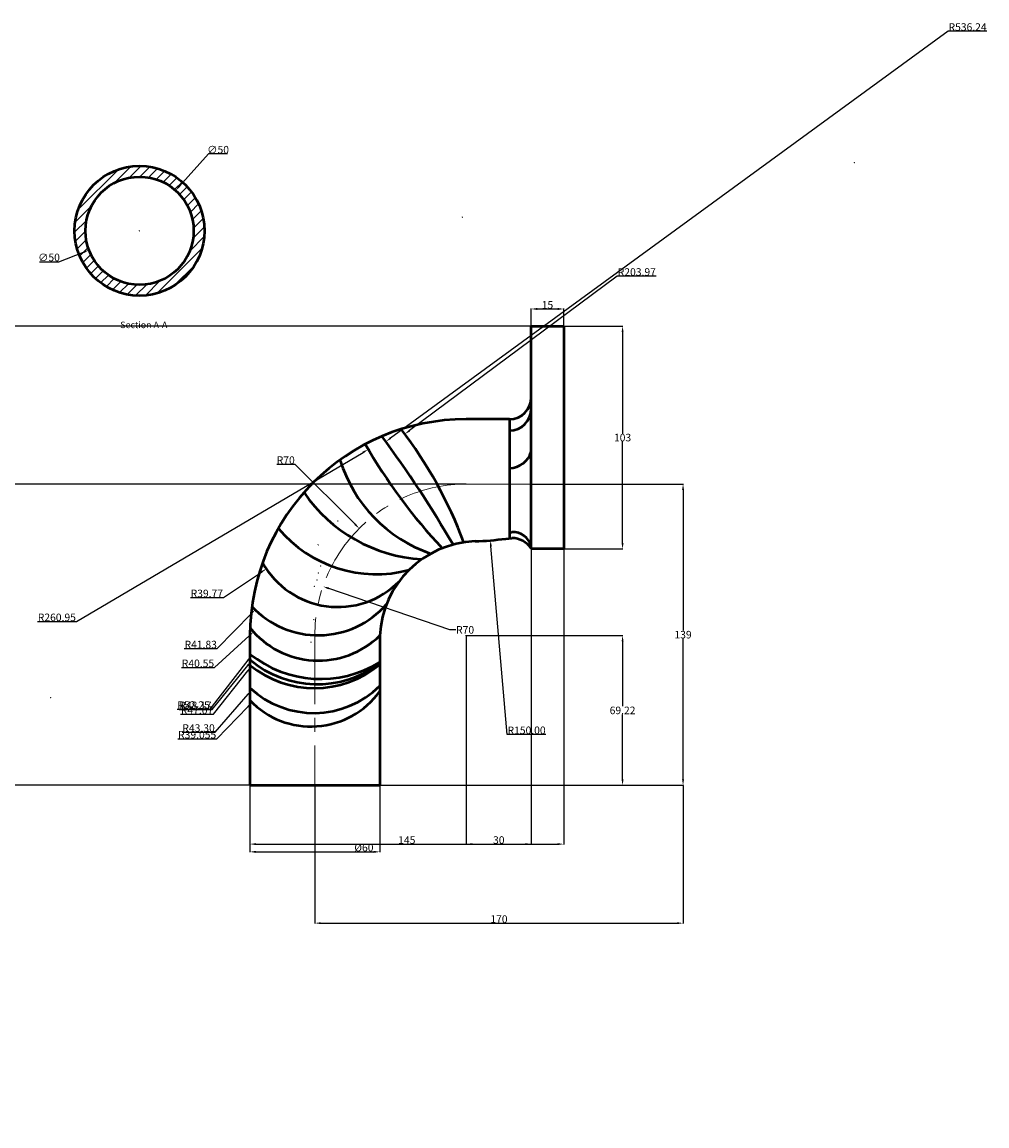
# Model space of a CAD drawing. Units: millimetres. Extents: x 795 to 1506, y 326 to 837.
# Tile 2 of 2: x 1060 to 1506, y 326 to 837. Entities that reach past the tile are written whole.
import ezdxf

# ---------------------------------------------------------------- set-up
doc = ezdxf.new("R2010")
doc.units = ezdxf.units.MM
doc.header["$MEASUREMENT"] = 0
doc.linetypes.add('CENTER', pattern=[50.8, 31.75, -6.35, 6.35, -6.35])
for name, color, linetype, lineweight in [('M-CNTR', 251, 'CENTER', 18), ('M-DIMS', 2, 'Continuous', 25), ('M-HATC', 8, 'Continuous', 18), ('M-OUTL', 7, 'Continuous', 50), ('M-TEXT', 7, 'Continuous', 25)]:
    doc.layers.add(name, color=color, linetype=linetype, lineweight=lineweight)
doc.styles.get("Standard").update_dxf_attribs({"font": 'arial.ttf'})
doc.dimstyles.get("Standard").update_dxf_attribs({"dimtxt": 3.5, "dimasz": 2.75, "dimexe": 0.18, "dimexo": 0.0625, "dimgap": 0.09, "dimtad": 1, "dimtih": 1, "dimtoh": 1, "dimdec": 0, "dimzin": 0, "dimdsep": 46, "dimtxsty": 'Standard', "dimcen": 0.09, "dimadec": 0, "dimazin": 0, "dimtfac": 1, "dimtdec": 0, "dimtofl": 0, "dimtmove": 0, "dimatfit": 3, "dimfxl": 1, "dimtolj": 1, "dimtzin": 0, "dimarcsym": 0})

# ---------------------------------------------------------------- blocks, each defined once
blk = doc.blocks.new('*D4')
at = {"layer": 'Defpoints', "color": 0, "transparency": 16777216}
for p in [(1295.11, 622.98), (1225.11, 483.77), (1365.27, 483.77)]:
    blk.add_point(p, dxfattribs=at)
at = {"layer": 'M-DIMS', "color": 0, "lineweight": -2, "transparency": 16777216}
for p, q in [((1295.17, 622.98), (1365.45, 622.98)), ((1365.27, 620.23), (1365.27, 555.25)), ((1365.27, 486.52), (1365.27, 551.5)), ((1225.17, 483.77), (1365.45, 483.77))]:
    blk.add_line(p, q, dxfattribs=at)
at = {"layer": 'M-DIMS', "color": 0, "transparency": 16777216}
for points in [[(1364.81, 620.23), (1365.72, 620.23), (1365.27, 622.98)], [(1364.81, 486.52), (1365.72, 486.52), (1365.27, 483.77)]]:
    blk.add_solid(points, dxfattribs=at)
at = {"layer": 'M-DIMS', "color": 0, "transparency": 16777216, "insert": (1365.27, 553.37), "char_height": 3.5, "attachment_point": 5}
blk.add_mtext('\\A1;139', dxfattribs=at)
blk = doc.blocks.new('*D5')
at = {"layer": 'Defpoints', "color": 0, "transparency": 16777216}
for p in [(1165.11, 483.77), (1225.11, 483.77), (1225.11, 452.98)]:
    blk.add_point(p, dxfattribs=at)
at = {"layer": 'M-DIMS', "color": 0, "lineweight": -2, "transparency": 16777216}
for p, q in [((1165.11, 483.7), (1165.11, 452.8)), ((1225.11, 483.7), (1225.11, 452.8)), ((1167.86, 452.98), (1222.36, 452.98))]:
    blk.add_line(p, q, dxfattribs=at)
at = {"layer": 'M-DIMS', "color": 0, "transparency": 16777216}
for points in [[(1167.86, 453.43), (1167.86, 452.52), (1165.11, 452.98)], [(1222.36, 453.43), (1222.36, 452.52), (1225.11, 452.98)]]:
    blk.add_solid(points, dxfattribs=at)
at = {"layer": 'M-DIMS', "color": 0, "transparency": 16777216, "insert": (1217.78, 454.95), "char_height": 3.5, "attachment_point": 5}
blk.add_mtext('\\A1;%%C60', dxfattribs=at)
blk = doc.blocks.new('*D6')
at = {"layer": 'Defpoints', "color": 0, "transparency": 16777216}
for p in [(1195.11, 483.77), (1365.27, 483.77), (1365.27, 420.02)]:
    blk.add_point(p, dxfattribs=at)
at = {"layer": 'M-DIMS', "color": 0, "lineweight": -2, "transparency": 16777216}
for p, q in [((1195.11, 483.7), (1195.11, 419.84)), ((1365.27, 483.7), (1365.27, 419.84)), ((1197.86, 420.02), (1362.52, 420.02))]:
    blk.add_line(p, q, dxfattribs=at)
at = {"layer": 'M-DIMS', "color": 0, "transparency": 16777216}
for points in [[(1197.86, 420.47), (1197.86, 419.56), (1195.11, 420.02)], [(1362.52, 420.47), (1362.52, 419.56), (1365.27, 420.02)]]:
    blk.add_solid(points, dxfattribs=at)
at = {"layer": 'M-DIMS', "color": 0, "transparency": 16777216, "insert": (1280.19, 421.89), "char_height": 3.5, "attachment_point": 5}
blk.add_mtext('\\A1;170', dxfattribs=at)
blk = doc.blocks.new('*D7')
at = {"layer": 'Defpoints', "color": 0, "transparency": 16777216}
for p in [(1310.11, 703.93), (1295.11, 695.98), (1310.11, 695.98)]:
    blk.add_point(p, dxfattribs=at)
at = {"layer": 'M-DIMS', "color": 0, "lineweight": -2, "transparency": 16777216}
for p, q in [((1295.11, 696.04), (1295.11, 704.11)), ((1297.86, 703.93), (1307.36, 703.93)), ((1310.11, 696.04), (1310.11, 704.11))]:
    blk.add_line(p, q, dxfattribs=at)
at = {"layer": 'M-DIMS', "color": 0, "transparency": 16777216}
for points in [[(1297.86, 704.39), (1297.86, 703.47), (1295.11, 703.93)], [(1307.36, 704.39), (1307.36, 703.47), (1310.11, 703.93)]]:
    blk.add_solid(points, dxfattribs=at)
at = {"layer": 'M-DIMS', "color": 0, "transparency": 16777216, "insert": (1302.61, 705.81), "char_height": 3.5, "attachment_point": 5}
blk.add_mtext('\\A1;15', dxfattribs=at)
blk = doc.blocks.new('*D16')
at = {"layer": 'Defpoints', "color": 0, "transparency": 16777216}
for p in [(1130.77, 758.69), (1097.42, 721.44)]:
    blk.add_point(p, dxfattribs=at)
at = {"layer": 'M-DIMS', "color": 0, "lineweight": -2, "transparency": 16777216}
for p, q in [((1145.89, 775.58), (1132.6, 760.74)), ((1154.79, 775.58), (1145.89, 775.58)), ((1114.01, 740.07), (1114.19, 740.07)), ((1114.1, 739.98), (1114.1, 740.16))]:
    blk.add_line(p, q, dxfattribs=at)
at = {"layer": 'M-DIMS', "color": 0, "transparency": 16777216}
blk.add_solid([(1132.26, 761.05), (1132.95, 760.44), (1130.77, 758.69)], dxfattribs=at)
at = {"layer": 'M-DIMS', "color": 0, "transparency": 16777216, "insert": (1150.39, 777.56), "char_height": 3.5, "attachment_point": 5}
blk.add_mtext('\\A1;∅50', dxfattribs=at)
blk = doc.blocks.new('*D17')
at = {"layer": 'Defpoints', "color": 0, "transparency": 16777216}
for p in [(1198.88, 575.65), (1265.11, 552.98)]:
    blk.add_point(p, dxfattribs=at)
at = {"layer": 'M-DIMS', "color": 0, "lineweight": -2, "transparency": 16777216}
for p, q in [((1257.53, 555.58), (1201.49, 574.76)), ((1260.28, 555.58), (1257.53, 555.58))]:
    blk.add_line(p, q, dxfattribs=at)
at = {"layer": 'M-DIMS', "color": 0, "transparency": 16777216}
blk.add_solid([(1201.63, 575.2), (1201.34, 574.33), (1198.88, 575.65)], dxfattribs=at)
at = {"layer": 'M-DIMS', "color": 0, "transparency": 16777216, "insert": (1264.54, 555.58), "char_height": 3.5, "attachment_point": 5}
blk.add_mtext('\\A1;R70', dxfattribs=at)
blk = doc.blocks.new('*D24')
at = {"layer": 'Defpoints', "color": 0, "transparency": 16777216}
for p in [(1310.11, 695.98), (1310.11, 592.98), (1337.31, 592.98)]:
    blk.add_point(p, dxfattribs=at)
at = {"layer": 'M-DIMS', "color": 0, "lineweight": -2, "transparency": 16777216}
for p, q in [((1310.17, 695.98), (1337.49, 695.98)), ((1337.31, 693.23), (1337.31, 646.36)), ((1337.31, 595.73), (1337.31, 642.6)), ((1310.17, 592.98), (1337.49, 592.98))]:
    blk.add_line(p, q, dxfattribs=at)
at = {"layer": 'M-DIMS', "color": 0, "transparency": 16777216}
for points in [[(1336.85, 693.23), (1337.77, 693.23), (1337.31, 695.98)], [(1336.85, 595.73), (1337.77, 595.73), (1337.31, 592.98)]]:
    blk.add_solid(points, dxfattribs=at)
at = {"layer": 'M-DIMS', "color": 0, "transparency": 16777216, "insert": (1337.31, 644.48), "char_height": 3.5, "attachment_point": 5}
blk.add_mtext('\\A1;103', dxfattribs=at)
blk = doc.blocks.new('*D25')
at = {"layer": 'Defpoints', "color": 0, "transparency": 16777216}
for p in [(1310.11, 695.98), (824.22, 622.98), (1265.11, 622.98)]:
    blk.add_point(p, dxfattribs=at)
at = {"layer": 'M-DIMS', "color": 0, "lineweight": -2, "transparency": 16777216}
for p, q in [((1310.05, 695.98), (824.04, 695.98)), ((824.22, 693.23), (824.22, 661.36)), ((824.22, 625.73), (824.22, 657.6)), ((1265.05, 622.98), (824.04, 622.98))]:
    blk.add_line(p, q, dxfattribs=at)
at = {"layer": 'M-DIMS', "color": 0, "transparency": 16777216}
for points in [[(823.76, 693.23), (824.68, 693.23), (824.22, 695.98)], [(823.76, 625.73), (824.68, 625.73), (824.22, 622.98)]]:
    blk.add_solid(points, dxfattribs=at)
at = {"layer": 'M-DIMS', "color": 0, "transparency": 16777216, "insert": (824.22, 659.48), "char_height": 3.5, "attachment_point": 5}
blk.add_mtext('\\A1;73', dxfattribs=at)
blk = doc.blocks.new('*D26')
at = {"layer": 'Defpoints', "color": 0, "transparency": 16777216}
for p in [(1310.11, 695.98), (1165.11, 483.77), (1310.11, 456.57)]:
    blk.add_point(p, dxfattribs=at)
at = {"layer": 'M-DIMS', "color": 0, "lineweight": -2, "transparency": 16777216}
for p, q in [((1310.11, 695.92), (1310.11, 456.39)), ((1165.11, 483.7), (1165.11, 456.39)), ((1167.86, 456.57), (1307.36, 456.57))]:
    blk.add_line(p, q, dxfattribs=at)
at = {"layer": 'M-DIMS', "color": 0, "transparency": 16777216}
for points in [[(1167.86, 457.02), (1167.86, 456.11), (1165.11, 456.57)], [(1307.36, 457.02), (1307.36, 456.11), (1310.11, 456.57)]]:
    blk.add_solid(points, dxfattribs=at)
at = {"layer": 'M-DIMS', "color": 0, "transparency": 16777216, "insert": (1237.61, 458.44), "char_height": 3.5, "attachment_point": 5}
blk.add_mtext('\\A1;145', dxfattribs=at)
blk = doc.blocks.new('*D27')
at = {"layer": 'Defpoints', "color": 0, "transparency": 16777216}
for p in [(824.22, 695.98), (1310.11, 695.98), (1165.11, 483.77)]:
    blk.add_point(p, dxfattribs=at)
at = {"layer": 'M-DIMS', "color": 0, "lineweight": -2, "transparency": 16777216}
for p, q in [((1310.05, 695.98), (824.04, 695.98)), ((824.22, 693.23), (824.22, 591.72)), ((824.22, 486.52), (824.22, 588.03)), ((1165.05, 483.77), (824.04, 483.77))]:
    blk.add_line(p, q, dxfattribs=at)
at = {"layer": 'M-DIMS', "color": 0, "transparency": 16777216}
for points in [[(823.76, 693.23), (824.68, 693.23), (824.22, 695.98)], [(823.76, 486.52), (824.68, 486.52), (824.22, 483.77)]]:
    blk.add_solid(points, dxfattribs=at)
at = {"layer": 'M-DIMS', "color": 0, "transparency": 16777216, "insert": (824.22, 589.87), "char_height": 3.5, "attachment_point": 5}
blk.add_mtext('\\A1;212.2', dxfattribs=at)
blk = doc.blocks.new('*D28')
at = {"layer": 'Defpoints', "color": 0, "transparency": 16777216}
for p in [(1265.11, 552.98), (1337.31, 552.98), (1225.11, 483.77)]:
    blk.add_point(p, dxfattribs=at)
at = {"layer": 'M-DIMS', "color": 0, "lineweight": -2, "transparency": 16777216}
for p, q in [((1265.17, 552.98), (1337.49, 552.98)), ((1337.31, 550.23), (1337.31, 520.25)), ((1337.31, 486.52), (1337.31, 516.5)), ((1225.17, 483.77), (1337.49, 483.77))]:
    blk.add_line(p, q, dxfattribs=at)
at = {"layer": 'M-DIMS', "color": 0, "transparency": 16777216}
for points in [[(1336.85, 550.23), (1337.77, 550.23), (1337.31, 552.98)], [(1336.85, 486.52), (1337.77, 486.52), (1337.31, 483.77)]]:
    blk.add_solid(points, dxfattribs=at)
at = {"layer": 'M-DIMS', "color": 0, "transparency": 16777216, "insert": (1337.31, 518.37), "char_height": 3.5, "attachment_point": 5}
blk.add_mtext('\\A1;69.22', dxfattribs=at)
blk = doc.blocks.new('*D29')
at = {"layer": 'Defpoints', "color": 0, "transparency": 16777216}
for p in [(1295.11, 592.98), (1265.11, 552.98), (1295.11, 456.57)]:
    blk.add_point(p, dxfattribs=at)
at = {"layer": 'M-DIMS', "color": 0, "lineweight": -2, "transparency": 16777216}
for p, q in [((1295.11, 592.92), (1295.11, 456.39)), ((1265.11, 552.92), (1265.11, 456.39)), ((1267.86, 456.57), (1292.36, 456.57))]:
    blk.add_line(p, q, dxfattribs=at)
at = {"layer": 'M-DIMS', "color": 0, "transparency": 16777216}
for points in [[(1267.86, 457.02), (1267.86, 456.11), (1265.11, 456.57)], [(1292.36, 457.02), (1292.36, 456.11), (1295.11, 456.57)]]:
    blk.add_solid(points, dxfattribs=at)
at = {"layer": 'M-DIMS', "color": 0, "transparency": 16777216, "insert": (1280.11, 458.44), "char_height": 3.5, "attachment_point": 5}
blk.add_mtext('\\A1;30', dxfattribs=at)
blk = doc.blocks.new('*D33')
at = {"layer": 'Defpoints', "color": 0, "transparency": 16777216}
for p in [(1215.61, 602.48), (1265.11, 552.98)]:
    blk.add_point(p, dxfattribs=at)
at = {"layer": 'M-DIMS', "color": 0, "lineweight": -2, "transparency": 16777216}
for p, q in [((1177.47, 632.18), (1185.91, 632.18)), ((1185.91, 632.18), (1213.67, 604.42)), ((1265.02, 552.98), (1265.2, 552.98)), ((1265.11, 552.89), (1265.11, 553.07))]:
    blk.add_line(p, q, dxfattribs=at)
at = {"layer": 'M-DIMS', "color": 0, "transparency": 16777216}
blk.add_solid([(1213.99, 604.75), (1213.34, 604.1), (1215.61, 602.48)], dxfattribs=at)
at = {"layer": 'M-DIMS', "color": 0, "transparency": 16777216, "insert": (1181.65, 634.05), "char_height": 3.5, "attachment_point": 5}
blk.add_mtext('\\A1;R70', dxfattribs=at)
blk = doc.blocks.new('*D34')
at = {"layer": 'Defpoints', "color": 0, "transparency": 16777216}
for p in [(1137.45, 749), (1090.74, 731.14)]:
    blk.add_point(p, dxfattribs=at)
at = {"layer": 'M-DIMS', "color": 0, "lineweight": -2, "transparency": 16777216}
for p, q in [((1114.01, 740.07), (1114.19, 740.07)), ((1114.1, 739.98), (1114.1, 740.16)), ((1076.73, 725.78), (1088.18, 730.16)), ((1067.83, 725.78), (1076.73, 725.78))]:
    blk.add_line(p, q, dxfattribs=at)
at = {"layer": 'M-DIMS', "color": 0, "transparency": 16777216}
blk.add_solid([(1088.01, 730.58), (1088.34, 729.73), (1090.74, 731.14)], dxfattribs=at)
at = {"layer": 'M-DIMS', "color": 0, "transparency": 16777216, "insert": (1072.24, 727.75), "char_height": 3.5, "attachment_point": 5}
blk.add_mtext('\\A1;∅50', dxfattribs=at)
blk = doc.blocks.new('*D36')
at = {"layer": 'Defpoints', "color": 0, "transparency": 16777216}
for p in [(1263.41, 746.42), (1276.23, 596.97)]:
    blk.add_point(p, dxfattribs=at)
at = {"layer": 'M-DIMS', "color": 0, "lineweight": -2, "transparency": 16777216}
for p, q in [((1263.32, 746.42), (1263.5, 746.42)), ((1263.41, 746.33), (1263.41, 746.51)), ((1283.92, 507.3), (1276.46, 594.23)), ((1301.88, 507.3), (1283.92, 507.3))]:
    blk.add_line(p, q, dxfattribs=at)
at = {"layer": 'M-DIMS', "color": 0, "transparency": 16777216}
blk.add_solid([(1276.92, 594.26), (1276.01, 594.19), (1276.23, 596.97)], dxfattribs=at)
at = {"layer": 'M-DIMS', "color": 0, "transparency": 16777216, "insert": (1292.95, 509.17), "char_height": 3.5, "attachment_point": 5}
blk.add_mtext('\\A1;R150.00', dxfattribs=at)
blk = doc.blocks.new('*D37')
at = {"layer": 'Defpoints', "color": 0, "transparency": 16777216}
for p in [(1236.69, 646.07), (1073.06, 524.3)]:
    blk.add_point(p, dxfattribs=at)
at = {"layer": 'M-DIMS', "color": 0, "lineweight": -2, "transparency": 16777216}
for p, q in [((1334.87, 719.13), (1238.9, 647.71)), ((1352.84, 719.13), (1334.87, 719.13)), ((1072.97, 524.3), (1073.15, 524.3)), ((1073.06, 524.21), (1073.06, 524.39))]:
    blk.add_line(p, q, dxfattribs=at)
at = {"layer": 'M-DIMS', "color": 0, "transparency": 16777216}
blk.add_solid([(1238.62, 648.08), (1239.17, 647.34), (1236.69, 646.07)], dxfattribs=at)
at = {"layer": 'M-DIMS', "color": 0, "transparency": 16777216, "insert": (1343.9, 721.01), "char_height": 3.5, "attachment_point": 5}
blk.add_mtext('\\A1;R203.97', dxfattribs=at)
blk = doc.blocks.new('*D38')
at = {"layer": 'Defpoints', "color": 0, "transparency": 16777216}
for p in [(1227.9, 642.63), (794.84, 326.38)]:
    blk.add_point(p, dxfattribs=at)
at = {"layer": 'M-DIMS', "color": 0, "lineweight": -2, "transparency": 16777216}
for p, q in [((1487.74, 832.38), (1230.12, 644.25)), ((1505.7, 832.38), (1487.74, 832.38)), ((794.75, 326.38), (794.93, 326.38)), ((794.84, 326.29), (794.84, 326.47))]:
    blk.add_line(p, q, dxfattribs=at)
at = {"layer": 'M-DIMS', "color": 0, "transparency": 16777216}
blk.add_solid([(1229.85, 644.62), (1230.39, 643.88), (1227.9, 642.63)], dxfattribs=at)
at = {"layer": 'M-DIMS', "color": 0, "transparency": 16777216, "insert": (1496.76, 834.26), "char_height": 3.5, "attachment_point": 5}
blk.add_mtext('\\A1;R536.24', dxfattribs=at)
blk = doc.blocks.new('*D39')
at = {"layer": 'Defpoints', "color": 0, "transparency": 16777216}
for p in [(1444.55, 771.58), (1219.77, 639.03)]:
    blk.add_point(p, dxfattribs=at)
at = {"layer": 'M-DIMS', "color": 0, "lineweight": -2, "transparency": 16777216}
for p, q in [((1444.46, 771.58), (1444.64, 771.58)), ((1444.55, 771.49), (1444.55, 771.67)), ((1084.91, 559.49), (1217.4, 637.63)), ((1066.91, 559.49), (1084.91, 559.49))]:
    blk.add_line(p, q, dxfattribs=at)
at = {"layer": 'M-DIMS', "color": 0, "transparency": 16777216}
blk.add_solid([(1217.17, 638.02), (1217.64, 637.23), (1219.77, 639.03)], dxfattribs=at)
at = {"layer": 'M-DIMS', "color": 0, "transparency": 16777216, "insert": (1075.87, 561.37), "char_height": 3.5, "attachment_point": 5}
blk.add_mtext('\\A1;R260.95', dxfattribs=at)
blk = doc.blocks.new('*D40')
at = {"layer": 'Defpoints', "color": 0, "transparency": 16777216}
for p in [(1205.74, 605.93), (1172.68, 583.82)]:
    blk.add_point(p, dxfattribs=at)
at = {"layer": 'M-DIMS', "color": 0, "lineweight": -2, "transparency": 16777216}
for p, q in [((1205.65, 605.93), (1205.83, 605.93)), ((1205.74, 605.84), (1205.74, 606.02)), ((1152.85, 570.56), (1170.4, 582.29)), ((1137.6, 570.56), (1152.85, 570.56))]:
    blk.add_line(p, q, dxfattribs=at)
at = {"layer": 'M-DIMS', "color": 0, "transparency": 16777216}
blk.add_solid([(1170.14, 582.68), (1170.65, 581.91), (1172.68, 583.82)], dxfattribs=at)
at = {"layer": 'M-DIMS', "color": 0, "transparency": 16777216, "insert": (1145.18, 572.44), "char_height": 3.5, "attachment_point": 5}
blk.add_mtext('\\A1;R39.77', dxfattribs=at)
blk = doc.blocks.new('*D41')
at = {"layer": 'Defpoints', "color": 0, "transparency": 16777216}
for p in [(1196.67, 594.93), (1167.52, 564.93)]:
    blk.add_point(p, dxfattribs=at)
at = {"layer": 'M-DIMS', "color": 0, "lineweight": -2, "transparency": 16777216}
for p, q in [((1196.58, 594.93), (1196.76, 594.93)), ((1196.67, 594.84), (1196.67, 595.02)), ((1150.03, 546.93), (1165.6, 562.96)), ((1134.78, 546.93), (1150.03, 546.93))]:
    blk.add_line(p, q, dxfattribs=at)
at = {"layer": 'M-DIMS', "color": 0, "transparency": 16777216}
blk.add_solid([(1165.28, 563.27), (1165.93, 562.64), (1167.52, 564.93)], dxfattribs=at)
at = {"layer": 'M-DIMS', "color": 0, "transparency": 16777216, "insert": (1142.36, 548.81), "char_height": 3.5, "attachment_point": 5}
blk.add_mtext('\\A1;R41.83', dxfattribs=at)
blk = doc.blocks.new('*D42')
at = {"layer": 'Defpoints', "color": 0, "transparency": 16777216}
for p in [(1196.73, 581.94), (1166.76, 554.63)]:
    blk.add_point(p, dxfattribs=at)
at = {"layer": 'M-DIMS', "color": 0, "lineweight": -2, "transparency": 16777216}
for p, q in [((1196.64, 581.94), (1196.82, 581.94)), ((1196.73, 581.85), (1196.73, 582.03)), ((1148.78, 538.24), (1164.73, 552.77)), ((1133.5, 538.24), (1148.78, 538.24))]:
    blk.add_line(p, q, dxfattribs=at)
at = {"layer": 'M-DIMS', "color": 0, "transparency": 16777216}
blk.add_solid([(1164.42, 553.11), (1165.03, 552.43), (1166.76, 554.63)], dxfattribs=at)
at = {"layer": 'M-DIMS', "color": 0, "transparency": 16777216, "insert": (1141.09, 540.11), "char_height": 3.5, "attachment_point": 5}
blk.add_mtext('\\A1;R40.55', dxfattribs=at)
blk = doc.blocks.new('*D43')
at = {"layer": 'Defpoints', "color": 0, "transparency": 16777216}
for p in [(1197.81, 585.18), (1165.91, 543.8)]:
    blk.add_point(p, dxfattribs=at)
at = {"layer": 'M-DIMS', "color": 0, "lineweight": -2, "transparency": 16777216}
for p, q in [((1197.72, 585.18), (1197.9, 585.18)), ((1197.81, 585.09), (1197.81, 585.27)), ((1146.76, 518.97), (1164.23, 541.62)), ((1131.49, 518.97), (1146.76, 518.97))]:
    blk.add_line(p, q, dxfattribs=at)
at = {"layer": 'M-DIMS', "color": 0, "transparency": 16777216}
blk.add_solid([(1163.86, 541.9), (1164.59, 541.34), (1165.91, 543.8)], dxfattribs=at)
at = {"layer": 'M-DIMS', "color": 0, "transparency": 16777216, "insert": (1139.08, 520.85), "char_height": 3.5, "attachment_point": 5}
blk.add_mtext('\\A1;R52.25', dxfattribs=at)
blk = doc.blocks.new('*D44')
at = {"layer": 'Defpoints', "color": 0, "transparency": 16777216}
for p in [(1196.16, 578.65), (1165.8, 541.25)]:
    blk.add_point(p, dxfattribs=at)
at = {"layer": 'M-DIMS', "color": 0, "lineweight": -2, "transparency": 16777216}
for p, q in [((1196.07, 578.65), (1196.25, 578.65)), ((1196.16, 578.56), (1196.16, 578.74)), ((1147.59, 518.81), (1164.07, 539.11)), ((1132.34, 518.81), (1147.59, 518.81))]:
    blk.add_line(p, q, dxfattribs=at)
at = {"layer": 'M-DIMS', "color": 0, "transparency": 16777216}
blk.add_solid([(1163.71, 539.4), (1164.43, 538.83), (1165.8, 541.25)], dxfattribs=at)
at = {"layer": 'M-DIMS', "color": 0, "transparency": 16777216, "insert": (1139.92, 520.69), "char_height": 3.5, "attachment_point": 5}
blk.add_mtext('\\A1;R48.17', dxfattribs=at)
blk = doc.blocks.new('*D45')
at = {"layer": 'Defpoints', "color": 0, "transparency": 16777216}
for p in [(1194.92, 575.75), (1165.8, 538.76)]:
    blk.add_point(p, dxfattribs=at)
at = {"layer": 'M-DIMS', "color": 0, "lineweight": -2, "transparency": 16777216}
for p, q in [((1194.83, 575.75), (1195.01, 575.75)), ((1194.92, 575.66), (1194.92, 575.84)), ((1148.33, 516.57), (1164.1, 536.6)), ((1133.08, 516.57), (1148.33, 516.57))]:
    blk.add_line(p, q, dxfattribs=at)
at = {"layer": 'M-DIMS', "color": 0, "transparency": 16777216}
blk.add_solid([(1163.74, 536.88), (1164.46, 536.32), (1165.8, 538.76)], dxfattribs=at)
at = {"layer": 'M-DIMS', "color": 0, "transparency": 16777216, "insert": (1140.66, 518.44), "char_height": 3.5, "attachment_point": 5}
blk.add_mtext('\\A1;R47.07', dxfattribs=at)
blk = doc.blocks.new('*D46')
at = {"layer": 'Defpoints', "color": 0, "transparency": 16777216}
for p in [(1194.65, 560.46), (1166.14, 527.87)]:
    blk.add_point(p, dxfattribs=at)
at = {"layer": 'M-DIMS', "color": 0, "lineweight": -2, "transparency": 16777216}
for p, q in [((1194.56, 560.46), (1194.74, 560.46)), ((1194.65, 560.37), (1194.65, 560.55)), ((1149.03, 508.33), (1164.33, 525.81)), ((1133.79, 508.33), (1149.03, 508.33))]:
    blk.add_line(p, q, dxfattribs=at)
at = {"layer": 'M-DIMS', "color": 0, "transparency": 16777216}
blk.add_solid([(1163.98, 526.11), (1164.67, 525.5), (1166.14, 527.87)], dxfattribs=at)
at = {"layer": 'M-DIMS', "color": 0, "transparency": 16777216, "insert": (1141.37, 510.2), "char_height": 3.5, "attachment_point": 5}
blk.add_mtext('\\A1;R43.30', dxfattribs=at)
blk = doc.blocks.new('*D47')
at = {"layer": 'Defpoints', "color": 0, "transparency": 16777216}
for p in [(1193.38, 549.97), (1166.11, 522.02)]:
    blk.add_point(p, dxfattribs=at)
at = {"layer": 'M-DIMS', "color": 0, "lineweight": -2, "transparency": 16777216}
for p, q in [((1193.29, 549.97), (1193.47, 549.97)), ((1193.38, 549.88), (1193.38, 550.06)), ((1149.75, 505.24), (1164.19, 520.05)), ((1131.75, 505.24), (1149.75, 505.24))]:
    blk.add_line(p, q, dxfattribs=at)
at = {"layer": 'M-DIMS', "color": 0, "transparency": 16777216}
blk.add_solid([(1163.86, 520.37), (1164.52, 519.73), (1166.11, 522.02)], dxfattribs=at)
at = {"layer": 'M-DIMS', "color": 0, "transparency": 16777216, "insert": (1140.71, 507.12), "char_height": 3.5, "attachment_point": 5}
blk.add_mtext('\\A1;R39.055', dxfattribs=at)

msp = doc.modelspace()

# ---------------------------------------------------------------- hatches: boundary and pattern name
at = {"layer": 'M-HATC'}
h = msp.add_hatch(dxfattribs=at)
h.set_pattern_fill('ANSI31', color=256, scale=25)
h.paths.add_polyline_path([(1144.0954, 740.0665, 1), (1084.0954, 740.0665, 1)])
h.paths.add_polyline_path([(1089.0954, 740.0665, -1), (1139.0954, 740.0665, -1)], flags=16)

# ---------------------------------------------------------------- linework, layer by layer
at = {"layer": 'M-CNTR'}
msp.add_lwpolyline([(1295.1104, 622.9815), (1265.1104, 622.9815, 0.41421356), (1195.1104, 552.9815), (1195.1104, 483.7661)], format="xyb", dxfattribs=at)
at = {"layer": 'M-OUTL'}
for p, q in [((1295.1104, 695.9815), (1310.1104, 695.9815)), ((1295.1104, 592.9815), (1295.1104, 695.9815)), ((1310.1104, 695.9815), (1310.1104, 592.9815)), ((1285.1104, 652.9815), (1265.1104, 652.9815)), ((1285.1104, 652.9815), (1285.1104, 597.9204)), ((1295.1104, 622.9815), (1295.1104, 652.9815)), ((1295.1104, 592.9815), (1295.1104, 622.9815)), ((1295.1104, 592.9815), (1295.1104, 602.9815)), ((1283.291, 597.7404), (1286.2034, 598.0285)), ((1285.1104, 600.679), (1286.2034, 600.7871)), ((1261.474, 595.5825), (1261.4784, 595.583)), ((1310.1104, 592.9815), (1295.1104, 592.9815)), ((1165.1104, 552.9815), (1165.1104, 483.7661)), ((1225.1104, 552.9815), (1225.1104, 483.7661)), ((1165.1104, 483.7661), (1225.1104, 483.7661))]:
    msp.add_line(p, q, dxfattribs=at)
for radius in [30, 25]:
    msp.add_circle((1114.0954, 740.0665), radius, dxfattribs=at)
for centre, radius, start, end in [((1285.1104, 662.9815), 10, 270, 0), ((1285.1104, 657.7744), 10, 270, 0), ((1265.1104, 552.9815), 100, 90, 180), ((1073.0576, 524.2991), 203.9686, 20.59223, 37.452786), ((794.8393, 326.3773), 536.245, 30.05935, 36.462283), ((1444.5474, 771.5822), 260.9495, 209.926584, 223.087569), ((1284.7749, 641.1665), 10.8151, 271.777545, 342.872399), ((1270.5365, 653.9491), 66.8125, 197.22509, 250.898635), ((1248.6085, 658.8273), 70.713, 214.167359, 266.7048), ((1223.4988, 640.2813), 58.9508, 219.84524, 284.90172), ((1263.4056, 746.4165), 150, 272.190108, 277.618091), ((1286.6851, 592.1502), 8.6503, 13.095727, 93.192284), ((1286.1223, 587.1873), 10.8414, 33.99892, 89.571796), ((1270.8895, 550.7249), 45.8346, 92.190108, 177.178057), ((1205.7449, 605.9298), 39.7705, 208.977116, 315.354986), ((1196.6741, 594.9269), 41.8311, 222.883813, 318.938676), ((1196.7272, 581.9416), 40.5499, 218.904441, 314.423515), ((1197.8131, 585.1755), 52.252, 231.2543, 301.494533), ((1196.163, 578.6482), 48.1704, 229.861343, 306.937119), ((1194.9229, 575.7483), 47.0743, 230.705482, 309.88683), ((1194.6538, 560.4565), 43.2964, 226.972347, 314.703996), ((1193.3808, 549.9737), 39.0549, 223.625701, 324.334732)]:
    msp.add_arc(centre, radius, start, end, dxfattribs=at)

# ---------------------------------------------------------------- texts
at = {"layer": 'M-TEXT', "insert": (1105.1852, 698.0761), "char_height": 3, "attachment_point": 1}
msp.add_mtext_dynamic_manual_height_columns('Section A-A', width=25.407908, gutter_width=1, heights=[0], dxfattribs=at)

# ---------------------------------------------------------------- dimensions: what is measured, and where the dimension line sits
at = {"layer": 'M-DIMS'}
for center, mpoint, override, picture, middle in [((794.8393, 326.3773), (1227.9024, 642.6287), {"dimdec": 2, "dimlfac": 1, "dimrnd": 0, "dimzin": 0, "dimdsep": 46, "dimlunit": 2}, '*D38', (1496.7629, 832.3796)), ((1444.5474, 771.5822), (1219.7735, 639.0254), {"dimdec": 2, "dimlfac": 1, "dimrnd": 0, "dimzin": 0, "dimdsep": 46, "dimlunit": 2}, '*D39', (1075.8662, 559.4913)), ((1263.4056, 746.4165), (1276.229, 596.9656), {"dimdec": 2, "dimlfac": 1, "dimrnd": 0, "dimzin": 0, "dimdsep": 46, "dimlunit": 2}, '*D36', (1292.9469, 507.2951)), ((1073.0576, 524.2991), (1236.6893, 646.0688), {"dimdec": 2, "dimlfac": 1, "dimrnd": 0, "dimzin": 0, "dimdsep": 46, "dimlunit": 2}, '*D37', (1343.8981, 719.1306)), ((1265.1104, 552.9815), (1215.613, 602.479), {"dimdec": 0, "dimlfac": 1, "dimrnd": 0, "dimzin": 0, "dimdsep": 46, "dimlunit": 2}, '*D33', (1181.6489, 632.1775)), ((1205.7449, 605.9298), (1172.6844, 583.8233), {"dimdec": 2, "dimlfac": 1, "dimrnd": 0, "dimzin": 0, "dimdsep": 46, "dimlunit": 2}, '*D40', (1145.1779, 570.5594)), ((1196.6741, 594.9269), (1167.5213, 564.9277), {"dimdec": 2, "dimlfac": 1, "dimrnd": 0, "dimzin": 0, "dimdsep": 46, "dimlunit": 2}, '*D41', (1142.3594, 546.9281)), ((1197.8131, 585.1755), (1165.9059, 543.7967), {"dimdec": 2, "dimlfac": 1, "dimrnd": 0, "dimzin": 0, "dimdsep": 46, "dimlunit": 2}, '*D43', (1139.0783, 518.9695)), ((1196.7272, 581.9416), (1166.7578, 554.6262), {"dimdec": 2, "dimlfac": 1, "dimrnd": 0, "dimzin": 0, "dimdsep": 46, "dimlunit": 2}, '*D42', (1141.0929, 538.2369)), ((1196.163, 578.6482), (1165.8027, 541.2497), {"dimdec": 2, "dimlfac": 1, "dimrnd": 0, "dimzin": 0, "dimdsep": 46, "dimlunit": 2}, '*D44', (1139.9164, 518.8107)), ((1194.9229, 575.7483), (1165.8048, 538.7601), {"dimdec": 2, "dimlfac": 1, "dimrnd": 0, "dimzin": 0, "dimdsep": 46, "dimlunit": 2}, '*D45', (1140.6637, 516.5672)), ((1265.1104, 552.9815), (1198.8833, 575.6524), {"dimclrd": 0, "dimclre": 0, "dimclrt": 0}, '*D17', (1264.542, 555.5776)), ((1194.6538, 560.4565), (1166.1404, 527.8747), {"dimdec": 2, "dimlfac": 1, "dimrnd": 0, "dimzin": 0, "dimdsep": 46, "dimlunit": 2}, '*D46', (1141.3682, 508.3257)), ((1193.3808, 549.9737), (1166.1108, 522.0161), {"dimdec": 3, "dimlfac": 1, "dimrnd": 0, "dimzin": 0, "dimdsep": 46, "dimlunit": 2}, '*D47', (1140.7058, 505.2415))]:
    dim = msp.add_radius_dim(center=center, mpoint=mpoint, dimstyle='Standard', override=override, dxfattribs=at)
    dim.commit()
    dim.dimension.update_dxf_attribs({"geometry": picture, "text_midpoint": middle, "dimtype": 164})
for p1, p2, override, picture, middle in [((1097.4208, 721.4397), (1130.77, 758.6933), {"dimclrd": 0, "dimclre": 0, "dimclrt": 0}, '*D16', (1150.3853, 775.5842)), ((1137.4464, 748.9956), (1090.7444, 731.1374), {"dimdec": 0, "dimlfac": 1, "dimrnd": 0, "dimzin": 0, "dimdsep": 46, "dimlunit": 2}, '*D34', (1072.2389, 725.7799))]:
    dim = msp.add_diameter_dim_2p(p1=p1, p2=p2, dimstyle='Standard', override=override, dxfattribs=at)
    dim.commit()
    dim.dimension.update_dxf_attribs({"geometry": picture, "text_midpoint": middle, "dimtype": 163})
for base, p1, p2, override, picture, middle in [((1310.1104, 703.9288), (1295.1104, 695.9815), (1310.1104, 695.9815), {"dimclrd": 0, "dimclre": 0, "dimclrt": 0}, '*D7', (1302.6104, 705.8058)), ((1310.1104, 456.5661), (1165.1104, 483.7661), (1310.1104, 695.9815), {"dimdec": 0, "dimlfac": 1, "dimrnd": 0, "dimzin": 0, "dimdsep": 46, "dimlunit": 2}, '*D26', (1237.6104, 458.4431)), ((1295.1104, 456.5661), (1265.1104, 552.9815), (1295.1104, 592.9815), {"dimdec": 0, "dimlfac": 1, "dimrnd": 0, "dimzin": 0, "dimdsep": 46, "dimlunit": 2}, '*D29', (1280.1104, 458.4443)), ((1365.2652, 420.0165), (1195.1104, 483.7661), (1365.2652, 483.7661), {"dimclrd": 0, "dimclre": 0, "dimclrt": 0}, '*D6', (1280.1878, 421.8935))]:
    dim = msp.add_linear_dim(base=base, p1=p1, p2=p2, dimstyle='Standard', override=override, dxfattribs=at)
    dim.commit()
    dim.dimension.update_dxf_attribs({"geometry": picture, "text_midpoint": middle})
for base, p1, p2, override, picture, middle in [((824.2181, 695.9815), (1165.1104, 483.7661), (1310.1104, 695.9815), {"dimdec": 1, "dimlfac": 1, "dimrnd": 0, "dimzin": 0, "dimdsep": 46, "dimlunit": 2}, '*D27', (824.2181, 589.8738)), ((824.2181, 622.9815), (1310.1104, 695.9815), (1265.1104, 622.9815), {"dimdec": 0, "dimlfac": 1, "dimrnd": 0, "dimzin": 0, "dimdsep": 46, "dimlunit": 2}, '*D25', (824.2181, 659.4815)), ((1337.3104, 592.9815), (1310.1104, 695.9815), (1310.1104, 592.9815), {"dimdec": 0, "dimlfac": 1, "dimrnd": 0, "dimzin": 0, "dimdsep": 46, "dimlunit": 2}, '*D24', (1337.3104, 644.4815)), ((1365.2652, 483.7661), (1295.1104, 622.9815), (1225.1104, 483.7661), {"dimclrd": 0, "dimclre": 0, "dimclrt": 0}, '*D4', (1365.2652, 553.3738)), ((1337.3104, 552.9815), (1225.1104, 483.7661), (1265.1104, 552.9815), {"dimdec": 2, "dimlfac": 1, "dimrnd": 0, "dimzin": 0, "dimdsep": 46, "dimlunit": 2}, '*D28', (1337.3104, 518.3738))]:
    dim = msp.add_linear_dim(base=base, p1=p1, p2=p2, angle=90, dimstyle='Standard', override=override, dxfattribs=at)
    dim.commit()
    dim.dimension.update_dxf_attribs({"geometry": picture, "text_midpoint": middle})
dim = msp.add_linear_dim(base=(1225.1104, 452.9754), p1=(1165.1104, 483.7661), p2=(1225.1104, 483.7661), text='%%C<>', dimstyle='Standard', override={"dimjust": 2, "dimclrd": 0, "dimclre": 0, "dimclrt": 0, "dimtofl": 1}, dxfattribs=at)
dim.commit()
dim.dimension.update_dxf_attribs({"geometry": '*D5', "text_midpoint": (1217.7756, 454.9503)})

doc.saveas('drawing.dxf')
